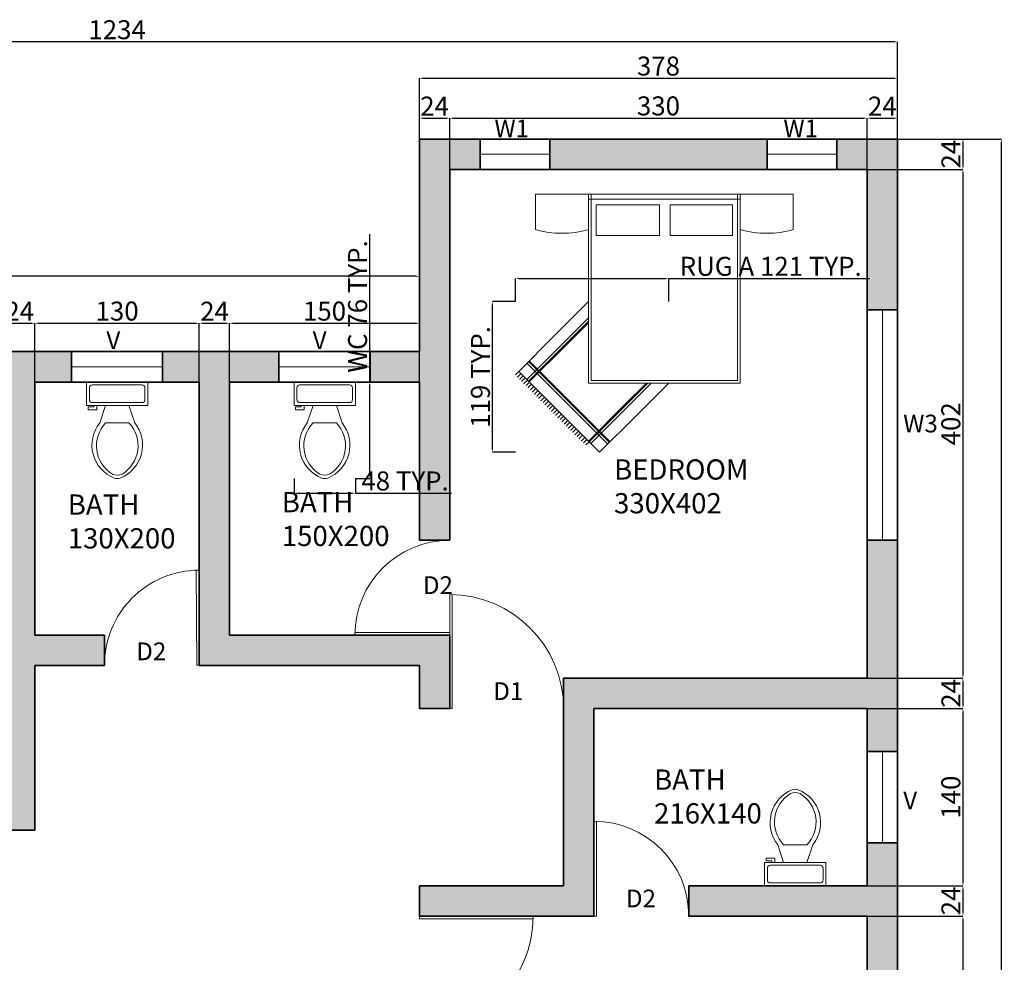
# Model space of a CAD drawing. Units: centimetres. Extents: x 2449 to 7478, y 778 to 2486.
# Tile 4 of 9: x 3118 to 3897, y 1732 to 2477. Entities that reach past the tile are written whole.
import ezdxf

# ---------------------------------------------------------------- set-up
doc = ezdxf.new("R2010")
doc.units = ezdxf.units.CM
for name, color, linetype, lineweight in [('A-ANNO-DIMS', 2, 'Continuous', 18), ('A-ANNO-TEXT', 7, 'Continuous', 18), ('A-AREA-IDEN', 7, 'Continuous', 18), ('A-DOOR', 4, 'Continuous', 18), ('A-FLOR-FIXT', 8, 'Continuous', 18), ('A-WALL', 7, 'Continuous', 35), ('A-WALL-PATT', 7, 'Continuous', 13), ('B-FURNITURE', 22, 'Continuous', 18), ('Win', 1, 'Continuous', 18)]:
    doc.layers.add(name, color=color, linetype=linetype, lineweight=lineweight)
doc.styles.get("Standard").update_dxf_attribs({"font": 'arial.ttf'})
doc.dimstyles.new('ISO-25', dxfattribs={"dimtxt": 15, "dimasz": 2.5, "dimexe": 0, "dimexo": 0, "dimgap": 0, "dimtad": 1, "dimtxsty": 'Standard', "dimcen": 2.5, "dimadec": 0, "dimazin": 0, "dimtfac": 1, "dimtmove": 0, "dimatfit": 3, "dimfxl": 1, "dimarcsym": 0})

# ---------------------------------------------------------------- blocks, each defined once
blk = doc.blocks.new('Toilet - top')
for p, q in [((9.5, -6), (9.5, -2)), ((-10, -8.5), (-8, -8.5)), ((-10, -9.5), (-10, -8.5)), ((-7, -9.5), (-10, -9.5)), ((-8, -8.5), (-8, -8)), ((-7, -8), (-7, -9.5)), ((-4, -8), (-6, -14)), ((4, -8), (6, -14)), ((4, -14), (-4, -14))]:
    blk.add_line(p, q)
blk.add_lwpolyline([(10.5, -8), (10.5, 0), (-10.5, 0), (-10.5, -8)], close=True)
for points in [[(-9.5, -2), (-9.5, -6)], [(8.5, -1), (-8.5, -1)], [(-8.5, -7), (8.5, -7)]]:
    blk.add_lwpolyline(points)
for centre, radius, start, end in [((-8.62, -1.88), 0.884, 81.8699, 188.1301), ((8.62, -1.88), 0.884, 351.8699, 98.1301), ((-8.62, -6.12), 0.884, 171.8699, 278.1301), ((8.62, -6.12), 0.884, 261.8699, 8.1301), ((3.52, -21.58), 12.17, 141.4691, 247.9714), ((4.2, -21.82), 11.33, 136.3677, 238.9468), ((-3.52, -21.58), 12.17, 292.0284, 38.5307), ((-4.2, -21.82), 11.33, 301.053, 43.6321), ((0, -27.88), 4, 245.7318, 294.2682), ((0, -29), 4, 254.8605, 285.1395)]:
    blk.add_arc(centre, radius, start, end)
blk = doc.blocks.new('A$C376C2187')
at = {"layer": 'B-FURNITURE'}
for p, q in [((-1.53, 1.82), (-1.53, 2.24)), ((-1.53, 2.24), (-0.9, 2.24)), ((-0.9, 0), (-0.9, 2.24)), ((-0.9, 2.24), (0.9, 2.24)), ((-0.9, 2.24), (-0.9, 1.82)), ((-0.87, 0.03), (-0.87, 2.24)), ((0.87, 2.24), (0.87, 0.03)), ((0.9, 2.24), (0.9, 0)), ((0.9, 1.82), (0.9, 2.24)), ((0.9, 2.24), (1.53, 2.24)), ((1.53, 2.24), (1.53, 1.82)), ((-0.9, 2.182), (0.9, 2.182)), ((-0.807, 2.112), (-0.057, 2.112)), ((-0.807, 1.749), (-0.807, 2.112)), ((-0.057, 2.112), (-0.057, 1.749)), ((0.069, 2.112), (0.807, 2.112)), ((0.069, 2.112), (0.069, 1.749)), ((0.807, 2.112), (0.807, 1.749)), ((-0.807, 1.749), (-0.057, 1.749)), ((0.069, 1.749), (0.807, 1.749)), ((0.9, 0), (-0.9, 0)), ((0.87, 0.03), (-0.87, 0.03))]:
    blk.add_line(p, q, dxfattribs=at)
for centre in [(-1.215, 2.926), (1.215, 2.926)]:
    blk.add_arc(centre, 1.15, 254.0965, 285.9035, dxfattribs=at)
blk = doc.blocks.new('*D19')
at = {"layer": 'A-ANNO-DIMS', "color": 0, "lineweight": -2, "transparency": 16777216}
for p, q in [((3106.09, 2190.34), (3106.09, 2236.78)), ((3108.59, 2236.78), (3127.59, 2236.78)), ((3130.09, 2190.34), (3130.09, 2236.78))]:
    blk.add_line(p, q, dxfattribs=at)
at = {"layer": 'A-ANNO-DIMS', "color": 0, "transparency": 16777216}
for points in [[(3108.59, 2237.19), (3108.59, 2236.36), (3106.09, 2236.78)], [(3127.59, 2237.19), (3127.59, 2236.36), (3130.09, 2236.78)]]:
    blk.add_solid(points, dxfattribs=at)
at = {"layer": 'Defpoints', "color": 0, "transparency": 16777216}
for p in [(3130.09, 2236.78), (3106.09, 2190.34), (3130.09, 2190.34)]:
    blk.add_point(p, dxfattribs=at)
at = {"layer": 'A-ANNO-DIMS', "color": 0, "transparency": 16777216, "insert": (3118.09, 2244.31), "char_height": 15, "attachment_point": 5}
blk.add_mtext('24', dxfattribs=at)
blk = doc.blocks.new('*D20')
at = {"layer": 'A-ANNO-DIMS', "color": 0, "lineweight": -2, "transparency": 16777216}
for p, q in [((3130.09, 2190.34), (3130.09, 2236.78)), ((3132.59, 2236.78), (3257.59, 2236.78)), ((3260.09, 2190.34), (3260.09, 2236.78))]:
    blk.add_line(p, q, dxfattribs=at)
at = {"layer": 'A-ANNO-DIMS', "color": 0, "transparency": 16777216}
for points in [[(3132.59, 2237.19), (3132.59, 2236.36), (3130.09, 2236.78)], [(3257.59, 2237.19), (3257.59, 2236.36), (3260.09, 2236.78)]]:
    blk.add_solid(points, dxfattribs=at)
at = {"layer": 'Defpoints', "color": 0, "transparency": 16777216}
for p in [(3260.09, 2236.78), (3130.09, 2190.34), (3260.09, 2190.34)]:
    blk.add_point(p, dxfattribs=at)
at = {"layer": 'A-ANNO-DIMS', "color": 0, "transparency": 16777216, "insert": (3195.09, 2244.44), "char_height": 15, "attachment_point": 5}
blk.add_mtext('130', dxfattribs=at)
blk = doc.blocks.new('*D21')
at = {"layer": 'A-ANNO-DIMS', "color": 0, "lineweight": -2, "transparency": 16777216}
for p, q in [((3260.09, 2190.34), (3260.09, 2236.78)), ((3262.59, 2236.78), (3281.59, 2236.78)), ((3284.09, 2190.34), (3284.09, 2236.78))]:
    blk.add_line(p, q, dxfattribs=at)
at = {"layer": 'A-ANNO-DIMS', "color": 0, "transparency": 16777216}
for points in [[(3262.59, 2237.19), (3262.59, 2236.36), (3260.09, 2236.78)], [(3281.59, 2237.19), (3281.59, 2236.36), (3284.09, 2236.78)]]:
    blk.add_solid(points, dxfattribs=at)
at = {"layer": 'Defpoints', "color": 0, "transparency": 16777216}
for p in [(3284.09, 2236.78), (3260.09, 2190.34), (3284.09, 2190.34)]:
    blk.add_point(p, dxfattribs=at)
at = {"layer": 'A-ANNO-DIMS', "color": 0, "transparency": 16777216, "insert": (3272.09, 2244.31), "char_height": 15, "attachment_point": 5}
blk.add_mtext('24', dxfattribs=at)
blk = doc.blocks.new('*D22')
at = {"layer": 'A-ANNO-DIMS', "color": 0, "lineweight": -2, "transparency": 16777216}
for p, q in [((3284.09, 2190.34), (3284.09, 2236.78)), ((3286.59, 2236.78), (3431.59, 2236.78)), ((3434.09, 2190.34), (3434.09, 2236.78))]:
    blk.add_line(p, q, dxfattribs=at)
at = {"layer": 'A-ANNO-DIMS', "color": 0, "transparency": 16777216}
for points in [[(3286.59, 2237.19), (3286.59, 2236.36), (3284.09, 2236.78)], [(3431.59, 2237.19), (3431.59, 2236.36), (3434.09, 2236.78)]]:
    blk.add_solid(points, dxfattribs=at)
at = {"layer": 'Defpoints', "color": 0, "transparency": 16777216}
for p in [(3434.09, 2236.78), (3284.09, 2190.34), (3434.09, 2190.34)]:
    blk.add_point(p, dxfattribs=at)
at = {"layer": 'A-ANNO-DIMS', "color": 0, "transparency": 16777216, "insert": (3359.09, 2244.43), "char_height": 15, "attachment_point": 5}
blk.add_mtext('150', dxfattribs=at)
blk = doc.blocks.new('*D23')
at = {"layer": 'A-ANNO-DIMS', "color": 0, "lineweight": -2, "transparency": 16777216}
for p, q in [((3434.09, 2382.34), (3434.09, 2398.87)), ((3436.59, 2398.87), (3455.59, 2398.87)), ((3458.09, 2358.34), (3458.09, 2398.87))]:
    blk.add_line(p, q, dxfattribs=at)
at = {"layer": 'A-ANNO-DIMS', "color": 0, "transparency": 16777216}
for points in [[(3436.59, 2399.29), (3436.59, 2398.46), (3434.09, 2398.87)], [(3455.59, 2399.29), (3455.59, 2398.46), (3458.09, 2398.87)]]:
    blk.add_solid(points, dxfattribs=at)
at = {"layer": 'Defpoints', "color": 0, "transparency": 16777216}
for p in [(3458.09, 2398.87), (3434.09, 2382.34), (3458.09, 2358.34)]:
    blk.add_point(p, dxfattribs=at)
at = {"layer": 'A-ANNO-DIMS', "color": 0, "transparency": 16777216, "insert": (3446.09, 2406.41), "char_height": 15, "attachment_point": 5}
blk.add_mtext('24', dxfattribs=at)
blk = doc.blocks.new('*D24')
at = {"layer": 'A-ANNO-DIMS', "color": 0, "lineweight": -2, "transparency": 16777216}
for p, q in [((3458.09, 2358.34), (3458.09, 2398.87)), ((3460.59, 2398.87), (3785.59, 2398.87)), ((3788.09, 2358.34), (3788.09, 2398.87))]:
    blk.add_line(p, q, dxfattribs=at)
at = {"layer": 'A-ANNO-DIMS', "color": 0, "transparency": 16777216}
for points in [[(3460.59, 2399.29), (3460.59, 2398.46), (3458.09, 2398.87)], [(3785.59, 2399.29), (3785.59, 2398.46), (3788.09, 2398.87)]]:
    blk.add_solid(points, dxfattribs=at)
at = {"layer": 'Defpoints', "color": 0, "transparency": 16777216}
for p in [(3788.09, 2398.87), (3458.09, 2358.34), (3788.09, 2358.34)]:
    blk.add_point(p, dxfattribs=at)
at = {"layer": 'A-ANNO-DIMS', "color": 0, "transparency": 16777216, "insert": (3623.09, 2406.54), "char_height": 15, "attachment_point": 5}
blk.add_mtext('330', dxfattribs=at)
blk = doc.blocks.new('*D25')
at = {"layer": 'A-ANNO-DIMS', "color": 0, "lineweight": -2, "transparency": 16777216}
for p, q in [((3788.09, 2358.34), (3788.09, 2398.87)), ((3790.59, 2398.87), (3809.59, 2398.87)), ((3812.09, 2382.34), (3812.09, 2398.87))]:
    blk.add_line(p, q, dxfattribs=at)
at = {"layer": 'A-ANNO-DIMS', "color": 0, "transparency": 16777216}
for points in [[(3790.59, 2399.29), (3790.59, 2398.46), (3788.09, 2398.87)], [(3809.59, 2399.29), (3809.59, 2398.46), (3812.09, 2398.87)]]:
    blk.add_solid(points, dxfattribs=at)
at = {"layer": 'Defpoints', "color": 0, "transparency": 16777216}
for p in [(3812.09, 2398.87), (3812.09, 2382.34), (3788.09, 2358.34)]:
    blk.add_point(p, dxfattribs=at)
at = {"layer": 'A-ANNO-DIMS', "color": 0, "transparency": 16777216, "insert": (3800.09, 2406.41), "char_height": 15, "attachment_point": 5}
blk.add_mtext('24', dxfattribs=at)
blk = doc.blocks.new('*D26')
at = {"layer": 'A-ANNO-DIMS', "color": 0, "lineweight": -2, "transparency": 16777216}
for p, q in [((2578.09, 2214.34), (2578.09, 2273.89)), ((3431.59, 2273.89), (2580.59, 2273.89)), ((3434.09, 2214.34), (3434.09, 2273.89))]:
    blk.add_line(p, q, dxfattribs=at)
at = {"layer": 'A-ANNO-DIMS', "color": 0, "transparency": 16777216}
for points in [[(2580.59, 2274.31), (2580.59, 2273.47), (2578.09, 2273.89)], [(3431.59, 2274.31), (3431.59, 2273.47), (3434.09, 2273.89)]]:
    blk.add_solid(points, dxfattribs=at)
at = {"layer": 'Defpoints', "color": 0, "transparency": 16777216}
for p in [(2578.09, 2273.89), (2578.09, 2214.34), (3434.09, 2214.34)]:
    blk.add_point(p, dxfattribs=at)
at = {"layer": 'A-ANNO-DIMS', "color": 0, "transparency": 16777216, "insert": (3006.09, 2281.55), "char_height": 15, "attachment_point": 5}
blk.add_mtext('856', dxfattribs=at)
blk = doc.blocks.new('*D27')
at = {"layer": 'A-ANNO-DIMS', "color": 0, "lineweight": -2, "transparency": 16777216}
for p, q in [((3434.09, 2382.34), (3434.09, 2430.38)), ((3436.59, 2430.38), (3809.59, 2430.38)), ((3812.09, 2382.34), (3812.09, 2430.38))]:
    blk.add_line(p, q, dxfattribs=at)
at = {"layer": 'A-ANNO-DIMS', "color": 0, "transparency": 16777216}
for points in [[(3436.59, 2430.79), (3436.59, 2429.96), (3434.09, 2430.38)], [(3809.59, 2430.79), (3809.59, 2429.96), (3812.09, 2430.38)]]:
    blk.add_solid(points, dxfattribs=at)
at = {"layer": 'Defpoints', "color": 0, "transparency": 16777216}
for p in [(3812.09, 2430.38), (3434.09, 2382.34), (3812.09, 2382.34)]:
    blk.add_point(p, dxfattribs=at)
at = {"layer": 'A-ANNO-DIMS', "color": 0, "transparency": 16777216, "insert": (3623.09, 2438.04), "char_height": 15, "attachment_point": 5}
blk.add_mtext('378', dxfattribs=at)
blk = doc.blocks.new('*D28')
at = {"layer": 'A-ANNO-DIMS', "color": 0, "lineweight": -2, "transparency": 16777216}
for p, q in [((2578.09, 2214.34), (2578.09, 2459.09)), ((3809.59, 2459.09), (2580.59, 2459.09)), ((3812.09, 2382.34), (3812.09, 2459.09))]:
    blk.add_line(p, q, dxfattribs=at)
at = {"layer": 'A-ANNO-DIMS', "color": 0, "transparency": 16777216}
for points in [[(2580.59, 2459.51), (2580.59, 2458.68), (2578.09, 2459.09)], [(3809.59, 2459.51), (3809.59, 2458.68), (3812.09, 2459.09)]]:
    blk.add_solid(points, dxfattribs=at)
at = {"layer": 'Defpoints', "color": 0, "transparency": 16777216}
for p in [(2578.09, 2459.09), (3812.09, 2382.34), (2578.09, 2214.34)]:
    blk.add_point(p, dxfattribs=at)
at = {"layer": 'A-ANNO-DIMS', "color": 0, "transparency": 16777216, "insert": (3195.09, 2466.76), "char_height": 15, "attachment_point": 5}
blk.add_mtext('1234', dxfattribs=at)
blk = doc.blocks.new('*D46')
at = {"layer": 'A-ANNO-DIMS', "color": 0, "lineweight": -2, "transparency": 16777216}
for p, q in [((3812.09, 2382.34), (3863.83, 2382.34)), ((3863.83, 2379.84), (3863.83, 2360.84)), ((3788.09, 2358.34), (3863.83, 2358.34))]:
    blk.add_line(p, q, dxfattribs=at)
at = {"layer": 'A-ANNO-DIMS', "color": 0, "transparency": 16777216}
for points in [[(3863.42, 2379.84), (3864.25, 2379.84), (3863.83, 2382.34)], [(3863.42, 2360.84), (3864.25, 2360.84), (3863.83, 2358.34)]]:
    blk.add_solid(points, dxfattribs=at)
at = {"layer": 'Defpoints', "color": 0, "transparency": 16777216}
for p in [(3812.09, 2382.34), (3788.09, 2358.34), (3863.83, 2358.34)]:
    blk.add_point(p, dxfattribs=at)
at = {"layer": 'A-ANNO-DIMS', "color": 0, "transparency": 16777216, "insert": (3856.3, 2370.34), "char_height": 15, "attachment_point": 5, "rotation": 90}
blk.add_mtext('24', dxfattribs=at)
blk = doc.blocks.new('*D47')
at = {"layer": 'A-ANNO-DIMS', "color": 0, "lineweight": -2, "transparency": 16777216}
for p, q in [((3788.09, 2358.34), (3863.83, 2358.34)), ((3863.83, 2355.84), (3863.83, 1958.84)), ((3788.09, 1956.34), (3863.83, 1956.34))]:
    blk.add_line(p, q, dxfattribs=at)
at = {"layer": 'A-ANNO-DIMS', "color": 0, "transparency": 16777216}
for points in [[(3863.42, 2355.84), (3864.25, 2355.84), (3863.83, 2358.34)], [(3863.42, 1958.84), (3864.25, 1958.84), (3863.83, 1956.34)]]:
    blk.add_solid(points, dxfattribs=at)
at = {"layer": 'Defpoints', "color": 0, "transparency": 16777216}
for p in [(3788.09, 2358.34), (3788.09, 1956.34), (3863.83, 1956.34)]:
    blk.add_point(p, dxfattribs=at)
at = {"layer": 'A-ANNO-DIMS', "color": 0, "transparency": 16777216, "insert": (3856.18, 2157.34), "char_height": 15, "attachment_point": 5, "rotation": 90}
blk.add_mtext('402', dxfattribs=at)
blk = doc.blocks.new('*D48')
at = {"layer": 'A-ANNO-DIMS', "color": 0, "lineweight": -2, "transparency": 16777216}
for p, q in [((3788.09, 1956.34), (3863.83, 1956.34)), ((3863.83, 1953.84), (3863.83, 1934.84)), ((3788.09, 1932.34), (3863.83, 1932.34))]:
    blk.add_line(p, q, dxfattribs=at)
at = {"layer": 'A-ANNO-DIMS', "color": 0, "transparency": 16777216}
for points in [[(3863.42, 1953.84), (3864.25, 1953.84), (3863.83, 1956.34)], [(3863.42, 1934.84), (3864.25, 1934.84), (3863.83, 1932.34)]]:
    blk.add_solid(points, dxfattribs=at)
at = {"layer": 'Defpoints', "color": 0, "transparency": 16777216}
for p in [(3788.09, 1956.34), (3788.09, 1932.34), (3863.83, 1932.34)]:
    blk.add_point(p, dxfattribs=at)
at = {"layer": 'A-ANNO-DIMS', "color": 0, "transparency": 16777216, "insert": (3856.3, 1944.34), "char_height": 15, "attachment_point": 5, "rotation": 90}
blk.add_mtext('24', dxfattribs=at)
blk = doc.blocks.new('*D49')
at = {"layer": 'A-ANNO-DIMS', "color": 0, "lineweight": -2, "transparency": 16777216}
for p, q in [((3788.09, 1932.34), (3863.83, 1932.34)), ((3863.83, 1929.84), (3863.83, 1794.84)), ((3788.09, 1792.34), (3863.83, 1792.34))]:
    blk.add_line(p, q, dxfattribs=at)
at = {"layer": 'A-ANNO-DIMS', "color": 0, "transparency": 16777216}
for points in [[(3863.42, 1929.84), (3864.25, 1929.84), (3863.83, 1932.34)], [(3863.42, 1794.84), (3864.25, 1794.84), (3863.83, 1792.34)]]:
    blk.add_solid(points, dxfattribs=at)
at = {"layer": 'Defpoints', "color": 0, "transparency": 16777216}
for p in [(3788.09, 1932.34), (3788.09, 1792.34), (3863.83, 1792.34)]:
    blk.add_point(p, dxfattribs=at)
at = {"layer": 'A-ANNO-DIMS', "color": 0, "transparency": 16777216, "insert": (3856.18, 1862.34), "char_height": 15, "attachment_point": 5, "rotation": 90}
blk.add_mtext('140', dxfattribs=at)
blk = doc.blocks.new('*D50')
at = {"layer": 'A-ANNO-DIMS', "color": 0, "lineweight": -2, "transparency": 16777216}
for p, q in [((3788.09, 1792.34), (3863.83, 1792.34)), ((3863.83, 1789.84), (3863.83, 1770.84)), ((3788.09, 1768.34), (3863.83, 1768.34))]:
    blk.add_line(p, q, dxfattribs=at)
at = {"layer": 'A-ANNO-DIMS', "color": 0, "transparency": 16777216}
for points in [[(3863.42, 1789.84), (3864.25, 1789.84), (3863.83, 1792.34)], [(3863.42, 1770.84), (3864.25, 1770.84), (3863.83, 1768.34)]]:
    blk.add_solid(points, dxfattribs=at)
at = {"layer": 'Defpoints', "color": 0, "transparency": 16777216}
for p in [(3788.09, 1792.34), (3788.09, 1768.34), (3863.83, 1768.34)]:
    blk.add_point(p, dxfattribs=at)
at = {"layer": 'A-ANNO-DIMS', "color": 0, "transparency": 16777216, "insert": (3856.3, 1780.34), "char_height": 15, "attachment_point": 5, "rotation": 90}
blk.add_mtext('24', dxfattribs=at)
blk = doc.blocks.new('*D51')
at = {"layer": 'A-ANNO-DIMS', "color": 0, "lineweight": -2, "transparency": 16777216}
for p, q in [((3788.09, 1768.34), (3863.83, 1768.34)), ((3863.83, 1765.84), (3863.83, 1430.84)), ((3788.09, 1428.34), (3863.83, 1428.34))]:
    blk.add_line(p, q, dxfattribs=at)
at = {"layer": 'A-ANNO-DIMS', "color": 0, "transparency": 16777216}
for points in [[(3863.42, 1765.84), (3864.25, 1765.84), (3863.83, 1768.34)], [(3863.42, 1430.84), (3864.25, 1430.84), (3863.83, 1428.34)]]:
    blk.add_solid(points, dxfattribs=at)
at = {"layer": 'Defpoints', "color": 0, "transparency": 16777216}
for p in [(3788.09, 1768.34), (3788.09, 1428.34), (3863.83, 1428.34)]:
    blk.add_point(p, dxfattribs=at)
at = {"layer": 'A-ANNO-DIMS', "color": 0, "transparency": 16777216, "insert": (3856.17, 1598.34), "char_height": 15, "attachment_point": 5, "rotation": 90}
blk.add_mtext('340', dxfattribs=at)
blk = doc.blocks.new('*D58')
at = {"layer": 'A-ANNO-DIMS', "color": 0, "lineweight": -2, "transparency": 16777216}
for p, q in [((3812.09, 2382.34), (3894.34, 2382.34)), ((3894.34, 1022.84), (3894.34, 2379.84)), ((3812.09, 1020.34), (3894.34, 1020.34))]:
    blk.add_line(p, q, dxfattribs=at)
at = {"layer": 'A-ANNO-DIMS', "color": 0, "transparency": 16777216}
for points in [[(3893.92, 2379.84), (3894.76, 2379.84), (3894.34, 2382.34)], [(3893.92, 1022.84), (3894.76, 1022.84), (3894.34, 1020.34)]]:
    blk.add_solid(points, dxfattribs=at)
at = {"layer": 'Defpoints', "color": 0, "transparency": 16777216}
for p in [(3812.09, 2382.34), (3894.34, 2382.34), (3812.09, 1020.34)]:
    blk.add_point(p, dxfattribs=at)
at = {"layer": 'A-ANNO-DIMS', "color": 0, "transparency": 16777216, "insert": (3886.68, 1701.34), "char_height": 15, "attachment_point": 5, "rotation": 90}
blk.add_mtext('1362', dxfattribs=at)
blk = doc.blocks.new('3')
for p, q in [((5936.31, 1821.57), (5936.31, 1746.57)), ((5938.31, 1821.57), (5938.31, 1746.57)), ((5938.31, 1746.57), (5936.31, 1746.57))]:
    blk.add_line(p, q)
blk.add_arc((5936.31, 1746.57), 75, 0, 90)
blk = doc.blocks.new('2')
for p, q in [((5717.35, 1812.71), (5717.35, 1722.71)), ((5719.35, 1812.71), (5719.35, 1722.71)), ((5719.35, 1722.71), (5717.35, 1722.71))]:
    blk.add_line(p, q)
blk.add_arc((5717.35, 1722.71), 90, 0, 90)
blk = doc.blocks.new('RUG-FRINGED-A')
for p, q in [((57.64, 119.07), (31.14, 92.56)), ((37.52, 86.17), (57.64, 106.29)), ((38.88, 84.82), (57.64, 103.58)), ((39.46, 84.24), (57.64, 102.42)), ((2.52, 63.95), (31.14, 92.56)), ((37.52, 86.17), (8.91, 57.56)), ((38.88, 84.82), (10.26, 56.2)), ((39.46, 84.24), (10.84, 55.62)), ((72.85, 6.39), (8.91, 70.34)), ((74.21, 7.74), (10.26, 71.69)), ((74.79, 8.33), (10.84, 72.27)), ((2.62, 63.84), (0, 61.22)), ((66.47, 0), (2.52, 63.95)), ((4.3, 62.16), (1.68, 59.54)), ((5.98, 60.48), (3.36, 57.86)), ((7.66, 58.8), (5.04, 56.18)), ((9.34, 57.12), (6.72, 54.5)), ((11.02, 55.44), (8.4, 52.82)), ((103.41, 54.71), (86.2, 37.5)), ((104.58, 54.71), (86.78, 36.92)), ((107.29, 54.71), (88.14, 35.56)), ((95.08, 28.62), (121.18, 54.71)), ((12.7, 53.76), (10.08, 51.14)), ((14.38, 52.08), (11.76, 49.46)), ((16.06, 50.4), (13.44, 47.78)), ((17.74, 48.72), (15.12, 46.1)), ((19.42, 47.04), (16.8, 44.42)), ((21.1, 45.36), (18.48, 42.74)), ((22.78, 43.68), (20.16, 41.06)), ((24.46, 42), (21.84, 39.38)), ((26.14, 40.32), (23.52, 37.7)), ((27.82, 38.64), (25.2, 36.02)), ((29.5, 36.96), (26.88, 34.34)), ((31.18, 35.28), (28.56, 32.66)), ((32.86, 33.6), (30.24, 30.98)), ((34.54, 31.92), (31.92, 29.3)), ((57.58, 8.88), (86.2, 37.5)), ((58.16, 8.3), (86.78, 36.92)), ((59.52, 6.95), (88.14, 35.56)), ((36.22, 30.24), (33.6, 27.62)), ((37.9, 28.56), (35.28, 25.94)), ((39.58, 26.88), (36.96, 24.26)), ((41.26, 25.2), (38.64, 22.58)), ((42.94, 23.52), (40.32, 20.9)), ((95.08, 28.62), (66.47, 0)), ((44.62, 21.84), (42, 19.22)), ((46.3, 20.16), (43.68, 17.54)), ((47.98, 18.48), (45.36, 15.86)), ((49.66, 16.8), (47.04, 14.18)), ((51.34, 15.12), (48.72, 12.5)), ((53.02, 13.44), (50.4, 10.82)), ((54.7, 11.76), (52.08, 9.14)), ((56.38, 10.08), (53.76, 7.46)), ((58.07, 8.4), (55.44, 5.78))]:
    blk.add_line(p, q)
for centre in [(1.62, 59.48), (3.3, 57.8), (4.98, 56.12), (6.66, 54.44), (8.34, 52.76), (10.02, 51.08), (11.7, 49.4), (13.38, 47.72), (15.06, 46.04), (16.74, 44.36), (18.42, 42.68), (20.1, 41), (21.78, 39.32), (23.46, 37.64), (25.14, 35.96), (26.82, 34.28), (28.5, 32.6), (30.18, 30.92), (31.86, 29.24), (33.54, 27.56), (35.22, 25.88), (36.9, 24.2), (38.58, 22.52), (40.26, 20.84), (41.94, 19.16), (43.62, 17.48), (45.3, 15.8), (46.98, 14.12), (48.66, 12.44), (50.34, 10.76), (52.02, 9.08)]:
    blk.add_circle(centre, 0.0789)
blk = doc.blocks.new('*D78')
at = {"layer": 'A-ANNO-DIMS', "color": 0, "lineweight": -2, "transparency": 16777216}
for p, q in [((3394.91, 2190.34), (3394.91, 2307.2)), ((3383.46, 2190.34), (3394.91, 2190.34)), ((3394.91, 2116.53), (3394.91, 2187.84)), ((3383.46, 2114.03), (3394.91, 2114.03))]:
    blk.add_line(p, q, dxfattribs=at)
at = {"layer": 'A-ANNO-DIMS', "color": 0, "transparency": 16777216}
for points in [[(3394.49, 2187.84), (3395.33, 2187.84), (3394.91, 2190.34)], [(3394.49, 2116.53), (3395.33, 2116.53), (3394.91, 2114.03)]]:
    blk.add_solid(points, dxfattribs=at)
at = {"layer": 'Defpoints', "color": 0, "transparency": 16777216}
for p in [(3383.46, 2190.34), (3394.91, 2190.34), (3383.46, 2114.03)]:
    blk.add_point(p, dxfattribs=at)
at = {"layer": 'A-ANNO-DIMS', "color": 0, "transparency": 16777216, "insert": (3387.15, 2250.02), "char_height": 15, "attachment_point": 5, "rotation": 90}
blk.add_mtext('WC 76 TYP.', dxfattribs=at)
blk = doc.blocks.new('*D79')
at = {"layer": 'A-ANNO-DIMS', "color": 0, "lineweight": -2, "transparency": 16777216}
for p, q in [((3334.97, 2114.03), (3334.97, 2102.58)), ((3383.46, 2114.03), (3383.46, 2102.58)), ((3337.47, 2102.58), (3380.96, 2102.58)), ((3383.46, 2102.58), (3459.58, 2102.58))]:
    blk.add_line(p, q, dxfattribs=at)
at = {"layer": 'A-ANNO-DIMS', "color": 0, "transparency": 16777216}
for points in [[(3337.47, 2103), (3337.47, 2102.16), (3334.97, 2102.58)], [(3380.96, 2103), (3380.96, 2102.16), (3383.46, 2102.58)]]:
    blk.add_solid(points, dxfattribs=at)
at = {"layer": 'Defpoints', "color": 0, "transparency": 16777216}
for p in [(3334.97, 2114.03), (3383.46, 2114.03), (3383.46, 2102.58)]:
    blk.add_point(p, dxfattribs=at)
at = {"layer": 'A-ANNO-DIMS', "color": 0, "transparency": 16777216, "insert": (3422.77, 2110.24), "char_height": 15, "attachment_point": 5}
blk.add_mtext('48 TYP.', dxfattribs=at)
blk = doc.blocks.new('*D86')
at = {"layer": 'A-ANNO-DIMS', "color": 0, "lineweight": -2, "transparency": 16777216}
for p, q in [((3510.13, 2253.88), (3510.13, 2272.05)), ((3512.63, 2272.05), (3628.81, 2272.05)), ((3631.31, 2253.88), (3631.31, 2272.05)), ((3631.31, 2272.05), (3789.88, 2272.05))]:
    blk.add_line(p, q, dxfattribs=at)
at = {"layer": 'A-ANNO-DIMS', "color": 0, "transparency": 16777216}
for points in [[(3512.63, 2272.47), (3512.63, 2271.64), (3510.13, 2272.05)], [(3628.81, 2272.47), (3628.81, 2271.64), (3631.31, 2272.05)]]:
    blk.add_solid(points, dxfattribs=at)
at = {"layer": 'Defpoints', "color": 0, "transparency": 16777216}
for p in [(3631.31, 2272.05), (3510.13, 2253.88), (3631.31, 2253.88)]:
    blk.add_point(p, dxfattribs=at)
at = {"layer": 'A-ANNO-DIMS', "color": 0, "transparency": 16777216, "insert": (3711.85, 2279.81), "char_height": 15, "attachment_point": 5}
blk.add_mtext('RUG A 121 TYP.', dxfattribs=at)
blk = doc.blocks.new('*D87')
at = {"layer": 'A-ANNO-DIMS', "color": 0, "lineweight": -2, "transparency": 16777216}
for p, q in [((3510.13, 2253.88), (3491.95, 2253.88)), ((3491.95, 2137.31), (3491.95, 2251.38)), ((3510.13, 2134.81), (3491.95, 2134.81))]:
    blk.add_line(p, q, dxfattribs=at)
at = {"layer": 'A-ANNO-DIMS', "color": 0, "transparency": 16777216}
for points in [[(3491.54, 2251.38), (3492.37, 2251.38), (3491.95, 2253.88)], [(3491.54, 2137.31), (3492.37, 2137.31), (3491.95, 2134.81)]]:
    blk.add_solid(points, dxfattribs=at)
at = {"layer": 'Defpoints', "color": 0, "transparency": 16777216}
for p in [(3491.95, 2253.88), (3510.13, 2253.88), (3510.13, 2134.81)]:
    blk.add_point(p, dxfattribs=at)
at = {"layer": 'A-ANNO-DIMS', "color": 0, "transparency": 16777216, "insert": (3484.29, 2194.34), "char_height": 15, "attachment_point": 5, "rotation": 90}
blk.add_mtext('119 TYP.', dxfattribs=at)

msp = doc.modelspace()

# ---------------------------------------------------------------- hatches: boundary and pattern name
at = {"layer": 'A-WALL-PATT'}
h = msp.add_hatch(color=256, dxfattribs=at)
h.dxf.hatch_style = 1
h.paths.add_polyline_path([(3060.088, 1092.34), (2986.088, 1092.34), (2986.088, 1068.34), (3084.088, 1068.34), (3084.088, 1476.34), (3060.088, 1476.34)])
h.paths.add_polyline_path([(2706.088, 1167.34), (2730.088, 1167.34), (2730.088, 1377.34), (2706.088, 1377.34)])
h.paths.add_polyline_path([(2804.088, 1068.34), (2804.088, 1092.34), (2730.088, 1092.34), (2730.088, 1112.34), (2706.088, 1112.34), (2706.088, 1068.34)])
h.paths.add_polyline_path([(2730.088, 1551.34), (2706.088, 1551.34), (2706.088, 1432.34), (2730.088, 1432.34), (2730.088, 1452.34), (2970.088, 1452.34), (2970.088, 1476.34), (2730.088, 1476.34)])
h.paths.add_polyline_path([(3434.088, 1654.34), (3434.088, 1266.34), (3405.088, 1266.34), (3405.088, 1242.34), (3458.088, 1242.34), (3458.088, 1404.34), (3482.088, 1404.34), (3482.088, 1428.34), (3458.088, 1428.34), (3458.088, 1678.34), (3260.088, 1678.34), (3260.088, 1654.34)])
h.paths.add_polyline_path([(3223.088, 1266.34), (3194.088, 1266.34), (3194.088, 1242.34), (3223.088, 1242.34)])
h.paths.add_polyline_path([(3812.088, 1506.339), (3788.088, 1506.339), (3788.088, 1428.34), (3764.088, 1428.34), (3764.088, 1404.34), (3812.088, 1404.34)])
h.paths.add_polyline_path([(3709.088, 1404.34), (3709.088, 1428.34), (3537.088, 1428.34), (3537.088, 1404.34)])
h.paths.add_polyline_path([(3788.088, 1688.339), (3812.088, 1688.339), (3812.088, 1826.34), (3788.088, 1826.34), (3788.088, 1792.34), (3647.088, 1792.34), (3647.088, 1768.34), (3788.088, 1768.34)])
h.paths.add_polyline_path([(3788.088, 1956.34), (3548.088, 1956.34), (3548.088, 1792.34), (3434.088, 1792.34), (3434.088, 1768.34), (3572.088, 1768.34), (3572.088, 1932.34), (3788.088, 1932.34), (3788.088, 1898.34), (3812.088, 1898.34), (3812.088, 2065.339), (3788.088, 2065.339)])
h.paths.add_polyline_path([(3788.088, 2358.34), (3788.088, 2247.339), (3812.088, 2247.339), (3812.088, 2382.34), (3764.088, 2382.34), (3764.088, 2358.34)])
h.paths.add_polyline_path([(3537.088, 2382.34), (3537.088, 2358.34), (3709.088, 2358.34), (3709.088, 2382.34)])
h.paths.add_polyline_path([(3458.088, 2358.34), (3482.088, 2358.34), (3482.088, 2382.34), (3434.088, 2382.34), (3434.088, 2214.34), (3395.088, 2214.34), (3395.088, 2190.34), (3434.088, 2190.34), (3434.088, 2065.34), (3458.088, 2065.34)])
h.paths.add_polyline_path([(3231.088, 2214.34), (3231.088, 2190.34), (3260.088, 2190.34), (3260.088, 1966.34), (3434.088, 1966.34), (3434.088, 1932.34), (3458.088, 1932.34), (3458.088, 1990.34), (3284.088, 1990.34), (3284.088, 2190.34), (3323.088, 2190.34), (3323.088, 2214.34)])
h.paths.add_polyline_path([(3130.088, 2190.34), (3159.088, 2190.34), (3159.088, 2214.34), (3032.088, 2214.34), (3032.088, 2190.34), (3106.088, 2190.34), (3106.088, 1836.34), (3130.088, 1836.34), (3130.088, 1966.34), (3185.088, 1966.34), (3185.088, 1990.34), (3130.088, 1990.34)])
h.paths.add_polyline_path([(2738.088, 2214.34), (2738.088, 2190.34), (2752.088, 2190.34), (2752.088, 1935.34), (2776.088, 1935.34), (2776.088, 2190.34), (2850.088, 2190.34), (2850.088, 2214.34)])
h.paths.add_polyline_path([(2578.088, 2152.839), (2602.088, 2152.839), (2602.088, 2190.34), (2616.088, 2190.34), (2616.088, 2214.34), (2578.088, 2214.34)])
h.paths.add_polyline_path([(2578.088, 1935.34), (2602.088, 1935.34), (2602.088, 1970.839), (2578.088, 1970.839)])
h.paths.add_polyline_path([(2706.088, 1836.34), (2706.088, 1791.34), (2730.088, 1791.34), (2730.088, 1836.34), (3016.088, 1836.34), (3016.088, 1860.34), (2578.088, 1860.34), (2578.088, 1836.34)])

# ---------------------------------------------------------------- linework, layer by layer
at = {"layer": 'A-WALL'}
for p, q in [((3434.088, 2382.34), (3812.088, 2382.34)), ((3434.088, 2214.34), (3434.088, 2382.34)), ((3482.088, 2382.34), (3482.088, 2358.34)), ((3537.088, 2382.34), (3537.088, 2358.34)), ((3709.088, 2382.34), (3709.088, 2358.34)), ((3764.088, 2382.34), (3764.088, 2358.34)), ((3812.088, 2382.34), (3812.088, 1020.34)), ((3458.088, 2358.34), (3458.088, 2065.34)), ((3458.088, 2358.34), (3788.088, 2358.34)), ((3788.088, 2358.34), (3788.088, 1956.34)), ((3788.088, 2247.339), (3812.088, 2247.339)), ((2578.088, 2214.34), (3434.088, 2214.34)), ((3159.088, 2190.34), (3159.088, 2214.34)), ((3231.088, 2190.34), (3231.088, 2214.34)), ((3323.088, 2190.34), (3323.088, 2214.34)), ((3395.088, 2190.34), (3395.088, 2214.34)), ((3130.088, 2190.34), (3130.088, 1990.34)), ((3130.088, 2190.34), (3260.088, 2190.34)), ((3260.088, 2190.34), (3260.088, 1966.34)), ((3284.088, 2190.34), (3284.088, 1990.34)), ((3284.088, 2190.34), (3434.088, 2190.34)), ((3434.088, 2190.34), (3434.088, 2065.34)), ((3434.088, 2065.34), (3458.088, 2065.34)), ((3788.088, 2065.339), (3812.088, 2065.339)), ((3130.088, 1990.34), (3185.088, 1990.34)), ((3185.088, 1990.34), (3185.088, 1966.34)), ((3284.088, 1990.34), (3458.088, 1990.34)), ((3458.088, 1990.34), (3458.088, 1932.34)), ((3130.088, 1966.34), (3185.088, 1966.34)), ((3130.088, 1966.34), (3130.088, 1836.34)), ((3260.088, 1966.34), (3434.088, 1966.34)), ((3434.088, 1966.34), (3434.088, 1932.34)), ((3548.088, 1956.34), (3788.088, 1956.34)), ((3548.088, 1956.34), (3548.088, 1792.34)), ((3434.088, 1932.34), (3458.088, 1932.34)), ((3572.088, 1932.34), (3572.088, 1768.34)), ((3572.088, 1932.34), (3788.088, 1932.34)), ((3788.088, 1932.34), (3788.088, 1792.34)), ((3788.088, 1898.34), (3812.088, 1898.34)), ((3106.088, 1836.34), (3130.088, 1836.34)), ((3788.088, 1826.34), (3812.088, 1826.34)), ((3434.088, 1792.34), (3548.088, 1792.34)), ((3434.088, 1792.34), (3434.088, 1768.34)), ((3647.088, 1792.34), (3788.088, 1792.34)), ((3647.088, 1792.34), (3647.088, 1768.34)), ((3434.088, 1768.34), (3572.088, 1768.34)), ((3647.088, 1768.34), (3788.088, 1768.34)), ((3788.088, 1768.34), (3788.088, 1428.34))]:
    msp.add_line(p, q, dxfattribs=at)
at = {"layer": 'Win'}
for p, q in [((3482.088, 2370.34), (3537.088, 2370.34)), ((3709.088, 2370.34), (3764.088, 2370.34)), ((3800.088, 2247.339), (3800.088, 2065.339)), ((3231.088, 2202.34), (3159.088, 2202.34)), ((3395.088, 2202.34), (3323.088, 2202.34)), ((3800.088, 1898.34), (3800.088, 1826.34))]:
    msp.add_line(p, q, dxfattribs=at)

# ---------------------------------------------------------------- block references
at = {"layer": 'A-DOOR'}
for name, p, rotation in [('3', (5204.656, -3945.97), 90), ('2', (1711.374, 7485.689), 270)]:
    msp.add_blockref(name, p, dxfattribs=dict(at, rotation=rotation))
at = {"layer": 'A-DOOR', "xscale": -1, "rotation": 0.2708478329988573}
msp.add_blockref('3', (9204.587, 248.208), dxfattribs=at)
at = {"layer": 'A-DOOR'}
for name, p in [('2', (-2259.261, 209.625)), ('3', (-2364.221, 21.772))]:
    msp.add_blockref(name, p, dxfattribs=at)
at = {"layer": 'A-FLOR-FIXT', "xscale": 2.309305753348624, "yscale": 2.309305753348624, "zscale": 2.309305753348624}
for p in [(3195.215, 2190.34), (3359.215, 2190.34)]:
    msp.add_blockref('Toilet - top', p, dxfattribs=at)
at = {"layer": 'A-FLOR-FIXT', "xscale": -2.309305753348624, "yscale": 2.309305753348624, "zscale": 2.309305753348624, "rotation": 180}
msp.add_blockref('Toilet - top', (3731.258, 1792.34), dxfattribs=at)
at = {"layer": 'B-FURNITURE', "xscale": 66.63496932822166, "yscale": 66.63496932822166, "zscale": 66.63496932822166}
msp.add_blockref('A$C376C2187', (3627.738, 2189.525), dxfattribs=at)
at = {"layer": 'B-FURNITURE'}
msp.add_blockref('RUG-FRINGED-A', (3510.129, 2134.812), dxfattribs=at)

# ---------------------------------------------------------------- texts
at = {"layer": 'A-ANNO-TEXT', "char_height": 14, "attachment_point": 1}
for s, insert in [('{\\fTimes New Roman|b0|i0|c0|p18;\\PW1}', (3493.426, 2421.005)), ('{\\fTimes New Roman|b0|i0|c0|p18;\\PW1}', (3721.867, 2421.005)), ('{\\fTimes New Roman|b0|i0|c0|p18;\\P   V}', (3173.777, 2253.652)), ('{\\fTimes New Roman|b0|i0|c0|p18;\\P   V}', (3336.867, 2253.652)), ('{\\fTimes New Roman|b0|i0|c0|p18;\\PW3}', (3816.594, 2187.869)), ('{\\fTimes New Roman|b0|i0|c0|p18;\\PD2}', (3436.861, 2060.184)), ('{\\fTimes New Roman|b0|i0|c0|p18;\\PD2}', (3210.238, 2007.896)), ('{\\fTimes New Roman|b0|i0|c0|p18;\\PD1}', (3492.52, 1976.446)), ('{\\fTimes New Roman|b0|i0|c0|p18;\\PV}', (3816.594, 1890.156)), ('{\\fTimes New Roman|b0|i0|c0|p18;\\PD2}', (3597.378, 1812.646))]:
    msp.add_mtext_dynamic_manual_height_columns(s, width=211.90348, gutter_width=12.5, heights=[0], dxfattribs=dict(at, insert=insert))
at = {"layer": 'A-AREA-IDEN', "char_height": 16, "attachment_point": 1}
for s, insert in [('{\\fTimes New Roman|b0|i0|c0|p18;\\PBEDROOM           330X402}', (3587.983, 2155.913)), ('{\\fTimes New Roman|b0|i0|c0|p18;\\PBATH\\P150X200}', (3325.327, 2130.078)), ('{\\fTimes New Roman|b0|i0|c0|p18;\\PBATH\\P130X200}', (3156.092, 2128.174)), ('{\\fTimes New Roman|b0|i0|c0|p18;\\PBATH\\P216X140}', (3619.608, 1910.877))]:
    msp.add_mtext_dynamic_manual_height_columns(s, width=211.90348, gutter_width=12.5, heights=[0], dxfattribs=dict(at, insert=insert))

# ---------------------------------------------------------------- dimensions: what is measured, and where the dimension line sits
at = {"layer": 'A-ANNO-DIMS'}
for base, p1, p2, override, picture, middle in [((2578.088, 2459.093), (3812.088, 2382.34), (2578.088, 2214.34), {"dimclrd": 0, "dimclre": 0, "dimclrt": 0}, '*D28', (3195.088, 2466.756)), ((3812.088, 2430.375), (3434.088, 2382.34), (3812.088, 2382.34), {"dimclrd": 0, "dimclre": 0, "dimclrt": 0}, '*D27', (3623.088, 2438.039)), ((3458.088, 2398.875), (3434.088, 2382.34), (3458.088, 2358.34), {"dimclrd": 0, "dimclre": 0, "dimclrt": 0}, '*D23', (3446.088, 2406.405)), ((3788.088, 2398.875), (3458.088, 2358.34), (3788.088, 2358.34), {"dimclrd": 0, "dimclre": 0, "dimclrt": 0, "dimtmove": 1}, '*D24', (3623.088, 2406.538)), ((3812.088, 2398.875), (3788.088, 2358.34), (3812.088, 2382.34), {"dimclrd": 0, "dimclre": 0, "dimclrt": 0, "dimtmove": 1}, '*D25', (3800.088, 2406.405)), ((2578.088, 2273.89), (3434.088, 2214.34), (2578.088, 2214.34), {"dimclrd": 0, "dimclre": 0, "dimclrt": 0}, '*D26', (3006.088, 2281.548)), ((3130.088, 2236.775), (3106.088, 2190.34), (3130.088, 2190.34), {"dimclrd": 0, "dimclre": 0, "dimclrt": 0, "dimtmove": 1}, '*D19', (3118.088, 2244.306)), ((3260.088, 2236.775), (3130.088, 2190.34), (3260.088, 2190.34), {"dimclrd": 0, "dimclre": 0, "dimclrt": 0, "dimtmove": 1}, '*D20', (3195.088, 2244.439)), ((3284.088, 2236.775), (3260.088, 2190.34), (3284.088, 2190.34), {"dimclrd": 0, "dimclre": 0, "dimclrt": 0, "dimtmove": 1}, '*D21', (3272.088, 2244.306)), ((3434.088, 2236.775), (3284.088, 2190.34), (3434.088, 2190.34), {"dimclrd": 0, "dimclre": 0, "dimclrt": 0, "dimtmove": 1}, '*D22', (3359.088, 2244.434))]:
    dim = msp.add_linear_dim(base=base, p1=p1, p2=p2, dimstyle='ISO-25', override=override, dxfattribs=at)
    dim.commit()
    dim.dimension.update_dxf_attribs({"geometry": picture, "text_midpoint": middle})
for base, p1, p2, override, picture, middle in [((3863.835, 2358.34), (3812.088, 2382.34), (3788.088, 2358.34), {"dimclrd": 0, "dimclre": 0, "dimclrt": 0}, '*D46', (3856.304, 2370.34)), ((3894.34, 2382.34), (3812.088, 1020.34), (3812.088, 2382.34), {"dimclrd": 0, "dimclre": 0, "dimclrt": 0}, '*D58', (3886.676, 1701.34)), ((3863.835, 1956.34), (3788.088, 2358.34), (3788.088, 1956.34), {"dimclrd": 0, "dimclre": 0, "dimclrt": 0, "dimtmove": 1}, '*D47', (3856.176, 2157.34)), ((3863.835, 1932.34), (3788.088, 1956.34), (3788.088, 1932.34), {"dimclrd": 0, "dimclre": 0, "dimclrt": 0, "dimtmove": 1}, '*D48', (3856.304, 1944.34)), ((3863.835, 1792.34), (3788.088, 1932.34), (3788.088, 1792.34), {"dimclrd": 0, "dimclre": 0, "dimclrt": 0, "dimtmove": 1}, '*D49', (3856.176, 1862.34)), ((3863.835, 1768.34), (3788.088, 1792.34), (3788.088, 1768.34), {"dimclrd": 0, "dimclre": 0, "dimclrt": 0, "dimtmove": 1}, '*D50', (3856.304, 1780.34)), ((3863.835, 1428.34), (3788.088, 1768.34), (3788.088, 1428.34), {"dimclrd": 0, "dimclre": 0, "dimclrt": 0, "dimtmove": 1}, '*D51', (3856.171, 1598.34))]:
    dim = msp.add_linear_dim(base=base, p1=p1, p2=p2, angle=90, dimstyle='ISO-25', override=override, dxfattribs=at)
    dim.commit()
    dim.dimension.update_dxf_attribs({"geometry": picture, "text_midpoint": middle})
for base, p1, p2, text, picture, middle in [((3631.307, 2272.054), (3510.129, 2253.877), (3631.307, 2253.877), 'RUG A <> TYP.', '*D86', (3711.846, 2279.81)), ((3383.463, 2102.579), (3334.967, 2114.026), (3383.463, 2114.026), '<> TYP.', '*D79', (3422.772, 2110.237))]:
    dim = msp.add_linear_dim(base=base, p1=p1, p2=p2, text=text, dimstyle='ISO-25', override={"dimdec": 0, "dimlfac": 1, "dimrnd": 0, "dimzin": 0, "dimdsep": 46, "dimlunit": 2}, dxfattribs=at)
    dim.commit()
    dim.dimension.update_dxf_attribs({"geometry": picture, "text_midpoint": middle})
for base, p1, p2, text, picture, middle in [((3394.91, 2190.34), (3383.463, 2114.026), (3383.463, 2190.34), 'WC <> TYP.', '*D78', (3387.154, 2250.021)), ((3491.952, 2253.877), (3510.129, 2134.812), (3510.129, 2253.877), '<> TYP.', '*D87', (3484.294, 2194.345))]:
    dim = msp.add_linear_dim(base=base, p1=p1, p2=p2, angle=90, text=text, dimstyle='ISO-25', override={"dimdec": 0, "dimlfac": 1, "dimrnd": 0, "dimzin": 0, "dimdsep": 46, "dimlunit": 2}, dxfattribs=at)
    dim.commit()
    dim.dimension.update_dxf_attribs({"geometry": picture, "text_midpoint": middle})

doc.saveas('drawing.dxf')
